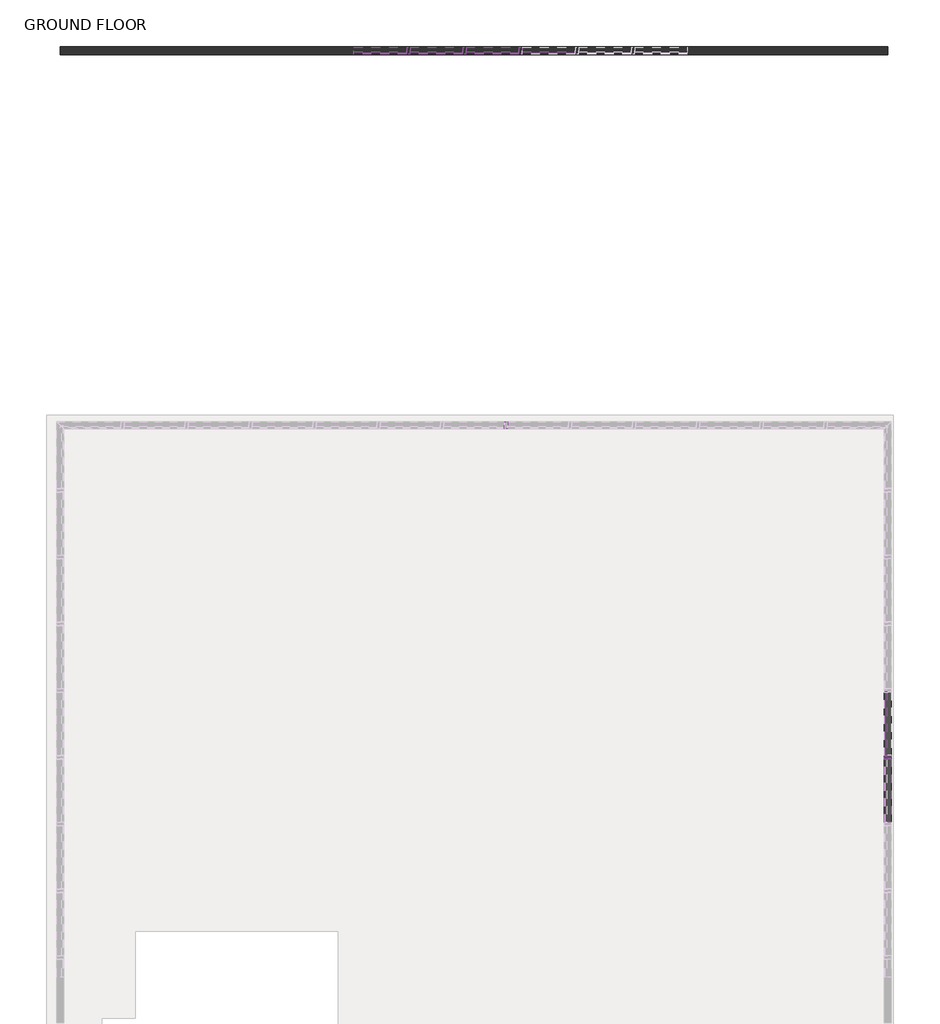
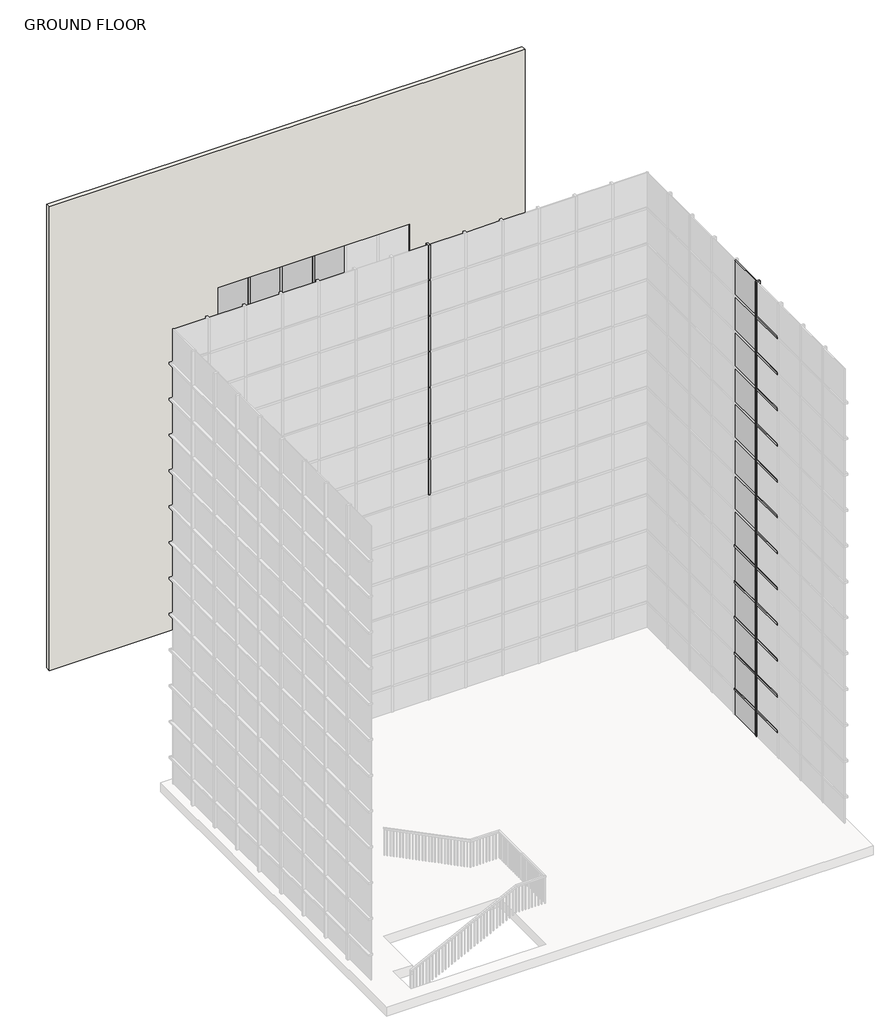
# One storey, part 11 of 16: 82 members, 45 plates, 1 wall.
"""IFC4 building model written with IfcOpenShell, lengths in millimetres."""

from ifc_helpers import new_model, si_unit, frame, origin, place, context, project, spatial, polyline, outline, extrude, transform, mapped, element, save
from components import member_b860638c, member_31fee25f, member_49b1bc66, member_76449a13, member_fdbefc00, member_3df3cfcf, member_368818a6, system_panel_glazed_49652e9e, system_panel_glazed_6a711426

model = new_model("IFC4")

# Units and contexts
model_context = context("Model", 3, world=origin())
ifc_project = project(units=[si_unit("LENGTHUNIT", "METRE", prefix="MILLI")], contexts=[model_context])

# Site, building, storey
site = spatial("IfcSite", under=ifc_project)
building = spatial("IfcBuilding", under=site)
storey = spatial("IfcBuildingStorey", under=building, Name="GROUND FLOOR", Elevation=0.0)

# Members
placement = place(None, origin())
member_shape = member_b860638c(model_context)
element("IfcMember", 1, ObjectType="Rectangular Mullion : 2.5\" x 5\" rectangular", at=placement, inside=storey, context=model_context, shape_type="MappedRepresentation", body=[
    mapped(member_shape, transform((5962.6982466, 315.5011968, 0.0), x_axis=(0.0, 1.0, 0.0), y_axis=(1.0, 0.0, 0.0), z_axis=(0.0, 0.0, -1.0))),
])
member_2_shape = member_31fee25f(model_context)
element("IfcMember", 2, ObjectType="Rectangular Mullion : 2.5\" x 5\" rectangular", at=placement, inside=storey, context=model_context, shape_type="MappedRepresentation", body=[
    mapped(member_2_shape, transform((5962.6982466, 315.5011968, 1168.8884615), x_axis=(0.0, 1.0, 0.0), y_axis=(1.0, 0.0, 0.0), z_axis=(0.0, 0.0, -1.0))),
])
element("IfcMember", 3, ObjectType="Rectangular Mullion : 2.5\" x 5\" rectangular", at=placement, inside=storey, context=model_context, shape_type="MappedRepresentation", body=[
    mapped(member_2_shape, transform((5962.6982466, 315.5011968, 2369.5269231), x_axis=(0.0, 1.0, 0.0), y_axis=(1.0, 0.0, 0.0), z_axis=(0.0, 0.0, -1.0))),
])
element("IfcMember", 4, ObjectType="Rectangular Mullion : 2.5\" x 5\" rectangular", at=placement, inside=storey, context=model_context, shape_type="MappedRepresentation", body=[
    mapped(member_2_shape, transform((5962.6982466, 315.5011968, 3570.1653846), x_axis=(0.0, 1.0, 0.0), y_axis=(1.0, 0.0, 0.0), z_axis=(0.0, 0.0, -1.0))),
])
element("IfcMember", 5, ObjectType="Rectangular Mullion : 2.5\" x 5\" rectangular", at=placement, inside=storey, context=model_context, shape_type="MappedRepresentation", body=[
    mapped(member_2_shape, transform((5962.6982466, 315.5011968, 4770.8038462), x_axis=(0.0, 1.0, 0.0), y_axis=(1.0, 0.0, 0.0), z_axis=(0.0, 0.0, -1.0))),
])
element("IfcMember", 6, ObjectType="Rectangular Mullion : 2.5\" x 5\" rectangular", at=placement, inside=storey, context=model_context, shape_type="MappedRepresentation", body=[
    mapped(member_2_shape, transform((5962.6982466, 315.5011968, 5971.4423077), x_axis=(0.0, 1.0, 0.0), y_axis=(1.0, 0.0, 0.0), z_axis=(0.0, 0.0, -1.0))),
])
element("IfcMember", 7, ObjectType="Rectangular Mullion : 2.5\" x 5\" rectangular", at=placement, inside=storey, context=model_context, shape_type="MappedRepresentation", body=[
    mapped(member_2_shape, transform((5962.6982466, 315.5011968, 7172.0807692), x_axis=(0.0, 1.0, 0.0), y_axis=(1.0, 0.0, 0.0), z_axis=(0.0, 0.0, -1.0))),
])
element("IfcMember", 8, ObjectType="Rectangular Mullion : 2.5\" x 5\" rectangular", at=placement, inside=storey, context=model_context, shape_type="MappedRepresentation", body=[
    mapped(member_2_shape, transform((5962.6982466, 315.5011968, 8372.7192308), x_axis=(0.0, 1.0, 0.0), y_axis=(1.0, 0.0, 0.0), z_axis=(0.0, 0.0, -1.0))),
])
element("IfcMember", 9, ObjectType="Rectangular Mullion : 2.5\" x 5\" rectangular", at=placement, inside=storey, context=model_context, shape_type="MappedRepresentation", body=[
    mapped(member_2_shape, transform((5962.6982466, 315.5011968, 9573.3576923), x_axis=(0.0, 1.0, 0.0), y_axis=(1.0, 0.0, 0.0), z_axis=(0.0, 0.0, -1.0))),
])
element("IfcMember", 10, ObjectType="Rectangular Mullion : 2.5\" x 5\" rectangular", at=placement, inside=storey, context=model_context, shape_type="MappedRepresentation", body=[
    mapped(member_2_shape, transform((5962.6982466, 315.5011968, 10773.9961538), x_axis=(0.0, 1.0, 0.0), y_axis=(1.0, 0.0, 0.0), z_axis=(0.0, 0.0, -1.0))),
])
element("IfcMember", 11, ObjectType="Rectangular Mullion : 2.5\" x 5\" rectangular", at=placement, inside=storey, context=model_context, shape_type="MappedRepresentation", body=[
    mapped(member_2_shape, transform((5962.6982466, 315.5011968, 11974.6346154), x_axis=(0.0, 1.0, 0.0), y_axis=(1.0, 0.0, 0.0), z_axis=(0.0, 0.0, -1.0))),
])
element("IfcMember", 12, ObjectType="Rectangular Mullion : 2.5\" x 5\" rectangular", at=placement, inside=storey, context=model_context, shape_type="MappedRepresentation", body=[
    mapped(member_2_shape, transform((5962.6982466, 315.5011968, 13175.2730769), x_axis=(0.0, 1.0, 0.0), y_axis=(1.0, 0.0, 0.0), z_axis=(0.0, 0.0, -1.0))),
])
element("IfcMember", 13, ObjectType="Rectangular Mullion : 2.5\" x 5\" rectangular", at=placement, inside=storey, context=model_context, shape_type="MappedRepresentation", body=[
    mapped(member_2_shape, transform((-998.3671381, 6370.2261968, 7172.0807692), x_axis=(-1.0, 0.0, 0.0), y_axis=(0.0, 1.0, 0.0), z_axis=(0.0, 0.0, -1.0))),
])
element("IfcMember", 14, ObjectType="Rectangular Mullion : 2.5\" x 5\" rectangular", at=placement, inside=storey, context=model_context, shape_type="MappedRepresentation", body=[
    mapped(member_2_shape, transform((-998.3671381, 6370.2261968, 8372.7192308), x_axis=(-1.0, 0.0, 0.0), y_axis=(0.0, 1.0, 0.0), z_axis=(0.0, 0.0, -1.0))),
])
element("IfcMember", 15, ObjectType="Rectangular Mullion : 2.5\" x 5\" rectangular", at=placement, inside=storey, context=model_context, shape_type="MappedRepresentation", body=[
    mapped(member_2_shape, transform((-998.3671381, 6370.2261968, 9573.3576923), x_axis=(-1.0, 0.0, 0.0), y_axis=(0.0, 1.0, 0.0), z_axis=(0.0, 0.0, -1.0))),
])
element("IfcMember", 16, ObjectType="Rectangular Mullion : 2.5\" x 5\" rectangular", at=placement, inside=storey, context=model_context, shape_type="MappedRepresentation", body=[
    mapped(member_2_shape, transform((-998.3671381, 6370.2261968, 10773.9961538), x_axis=(-1.0, 0.0, 0.0), y_axis=(0.0, 1.0, 0.0), z_axis=(0.0, 0.0, -1.0))),
])
element("IfcMember", 17, ObjectType="Rectangular Mullion : 2.5\" x 5\" rectangular", at=placement, inside=storey, context=model_context, shape_type="MappedRepresentation", body=[
    mapped(member_2_shape, transform((-998.3671381, 6370.2261968, 11974.6346154), x_axis=(-1.0, 0.0, 0.0), y_axis=(0.0, 1.0, 0.0), z_axis=(0.0, 0.0, -1.0))),
])
element("IfcMember", 18, ObjectType="Rectangular Mullion : 2.5\" x 5\" rectangular", at=placement, inside=storey, context=model_context, shape_type="MappedRepresentation", body=[
    mapped(member_2_shape, transform((-998.3671381, 6370.2261968, 13175.2730769), x_axis=(-1.0, 0.0, 0.0), y_axis=(0.0, 1.0, 0.0), z_axis=(0.0, 0.0, -1.0))),
])
element("IfcMember", 19, ObjectType="Rectangular Mullion : 2.5\" x 5\" rectangular", at=placement, inside=storey, context=model_context, shape_type="MappedRepresentation", body=[
    mapped(member_shape, transform((5962.6982466, 315.5011968, 14375.9115385), x_axis=(0.0, 1.0, 0.0), y_axis=(1.0, 0.0, 0.0), z_axis=(0.0, 0.0, -1.0))),
])
element("IfcMember", 20, ObjectType="Rectangular Mullion : 2.5\" x 5\" rectangular", at=placement, inside=storey, context=model_context, shape_type="MappedRepresentation", body=[
    mapped(member_shape, transform((-998.3671381, 6370.2261968, 14375.9115385), x_axis=(-1.0, 0.0, 0.0), y_axis=(0.0, 1.0, 0.0), z_axis=(0.0, 0.0, -1.0))),
])
member_3_shape = member_49b1bc66(model_context)
element("IfcMember", 21, ObjectType="Rectangular Mullion : 2.5\" x 5\" rectangular", at=placement, inside=storey, context=model_context, shape_type="MappedRepresentation", body=[
    mapped(member_3_shape, transform((5962.6982466, 283.7511968, 1168.8884615), x_axis=(0.0, 0.0, 1.0), y_axis=(1.0, 0.0, 0.0), z_axis=(0.0, 1.0, 0.0))),
])
element("IfcMember", 22, ObjectType="Rectangular Mullion : 2.5\" x 5\" rectangular", at=placement, inside=storey, context=model_context, shape_type="MappedRepresentation", body=[
    mapped(member_3_shape, transform((5962.6982466, 1501.0461967, 1168.8884615), x_axis=(0.0, 0.0, 1.0), y_axis=(1.0, 0.0, 0.0), z_axis=(0.0, 1.0, 0.0))),
])
element("IfcMember", 23, ObjectType="Rectangular Mullion : 2.5\" x 5\" rectangular", at=placement, inside=storey, context=model_context, shape_type="MappedRepresentation", body=[
    mapped(member_3_shape, transform((5962.6982466, 283.7511968, 2369.5269231), x_axis=(0.0, 0.0, 1.0), y_axis=(1.0, 0.0, 0.0), z_axis=(0.0, 1.0, 0.0))),
])
element("IfcMember", 24, ObjectType="Rectangular Mullion : 2.5\" x 5\" rectangular", at=placement, inside=storey, context=model_context, shape_type="MappedRepresentation", body=[
    mapped(member_3_shape, transform((5962.6982466, 1501.0461967, 2369.5269231), x_axis=(0.0, 0.0, 1.0), y_axis=(1.0, 0.0, 0.0), z_axis=(0.0, 1.0, 0.0))),
])
element("IfcMember", 25, ObjectType="Rectangular Mullion : 2.5\" x 5\" rectangular", at=placement, inside=storey, context=model_context, shape_type="MappedRepresentation", body=[
    mapped(member_3_shape, transform((5962.6982466, 283.7511968, 3570.1653846), x_axis=(0.0, 0.0, 1.0), y_axis=(1.0, 0.0, 0.0), z_axis=(0.0, 1.0, 0.0))),
])
element("IfcMember", 26, ObjectType="Rectangular Mullion : 2.5\" x 5\" rectangular", at=placement, inside=storey, context=model_context, shape_type="MappedRepresentation", body=[
    mapped(member_3_shape, transform((5962.6982466, 1501.0461967, 3570.1653846), x_axis=(0.0, 0.0, 1.0), y_axis=(1.0, 0.0, 0.0), z_axis=(0.0, 1.0, 0.0))),
])
element("IfcMember", 27, ObjectType="Rectangular Mullion : 2.5\" x 5\" rectangular", at=placement, inside=storey, context=model_context, shape_type="MappedRepresentation", body=[
    mapped(member_3_shape, transform((5962.6982466, 283.7511968, 4770.8038462), x_axis=(0.0, 0.0, 1.0), y_axis=(1.0, 0.0, 0.0), z_axis=(0.0, 1.0, 0.0))),
])
element("IfcMember", 28, ObjectType="Rectangular Mullion : 2.5\" x 5\" rectangular", at=placement, inside=storey, context=model_context, shape_type="MappedRepresentation", body=[
    mapped(member_3_shape, transform((5962.6982466, 1501.0461967, 4770.8038462), x_axis=(0.0, 0.0, 1.0), y_axis=(1.0, 0.0, 0.0), z_axis=(0.0, 1.0, 0.0))),
])
element("IfcMember", 29, ObjectType="Rectangular Mullion : 2.5\" x 5\" rectangular", at=placement, inside=storey, context=model_context, shape_type="MappedRepresentation", body=[
    mapped(member_3_shape, transform((5962.6982466, 283.7511968, 5971.4423077), x_axis=(0.0, 0.0, 1.0), y_axis=(1.0, 0.0, 0.0), z_axis=(0.0, 1.0, 0.0))),
])
element("IfcMember", 30, ObjectType="Rectangular Mullion : 2.5\" x 5\" rectangular", at=placement, inside=storey, context=model_context, shape_type="MappedRepresentation", body=[
    mapped(member_3_shape, transform((5962.6982466, 1501.0461967, 5971.4423077), x_axis=(0.0, 0.0, 1.0), y_axis=(1.0, 0.0, 0.0), z_axis=(0.0, 1.0, 0.0))),
])
element("IfcMember", 31, ObjectType="Rectangular Mullion : 2.5\" x 5\" rectangular", at=placement, inside=storey, context=model_context, shape_type="MappedRepresentation", body=[
    mapped(member_3_shape, transform((5962.6982466, 283.7511968, 7172.0807692), x_axis=(0.0, 0.0, 1.0), y_axis=(1.0, 0.0, 0.0), z_axis=(0.0, 1.0, 0.0))),
])
element("IfcMember", 32, ObjectType="Rectangular Mullion : 2.5\" x 5\" rectangular", at=placement, inside=storey, context=model_context, shape_type="MappedRepresentation", body=[
    mapped(member_3_shape, transform((5962.6982466, 283.7511968, 8372.7192308), x_axis=(0.0, 0.0, 1.0), y_axis=(1.0, 0.0, 0.0), z_axis=(0.0, 1.0, 0.0))),
])
element("IfcMember", 33, ObjectType="Rectangular Mullion : 2.5\" x 5\" rectangular", at=placement, inside=storey, context=model_context, shape_type="MappedRepresentation", body=[
    mapped(member_3_shape, transform((5962.6982466, 283.7511968, 9573.3576923), x_axis=(0.0, 0.0, 1.0), y_axis=(1.0, 0.0, 0.0), z_axis=(0.0, 1.0, 0.0))),
])
element("IfcMember", 34, ObjectType="Rectangular Mullion : 2.5\" x 5\" rectangular", at=placement, inside=storey, context=model_context, shape_type="MappedRepresentation", body=[
    mapped(member_3_shape, transform((5962.6982466, 283.7511968, 10773.9961538), x_axis=(0.0, 0.0, 1.0), y_axis=(1.0, 0.0, 0.0), z_axis=(0.0, 1.0, 0.0))),
])
element("IfcMember", 35, ObjectType="Rectangular Mullion : 2.5\" x 5\" rectangular", at=placement, inside=storey, context=model_context, shape_type="MappedRepresentation", body=[
    mapped(member_3_shape, transform((5962.6982466, 283.7511968, 11974.6346154), x_axis=(0.0, 0.0, 1.0), y_axis=(1.0, 0.0, 0.0), z_axis=(0.0, 1.0, 0.0))),
])
element("IfcMember", 36, ObjectType="Rectangular Mullion : 2.5\" x 5\" rectangular", at=placement, inside=storey, context=model_context, shape_type="MappedRepresentation", body=[
    mapped(member_3_shape, transform((5962.6982466, 283.7511968, 13175.2730769), x_axis=(0.0, 0.0, 1.0), y_axis=(1.0, 0.0, 0.0), z_axis=(0.0, 1.0, 0.0))),
])
element("IfcMember", 37, ObjectType="Rectangular Mullion : 2.5\" x 5\" rectangular", at=placement, inside=storey, context=model_context, shape_type="MappedRepresentation", body=[
    mapped(member_3_shape, transform((5962.6982466, 283.7511968, 14375.9115385), x_axis=(0.0, 0.0, 1.0), y_axis=(1.0, 0.0, 0.0), z_axis=(0.0, 1.0, 0.0))),
])
member_4_shape = member_76449a13(model_context)
element("IfcMember", 38, ObjectType="Rectangular Mullion : 2.5\" x 5\" rectangular", at=placement, inside=storey, context=model_context, shape_type="MappedRepresentation", body=[
    mapped(member_4_shape, transform((-765.2355616, 13200.7626438, 3045.6877023), x_axis=(0.0, 0.0, 1.0), y_axis=(0.0, -1.0, 0.0), z_axis=(1.0, 0.0, 0.0))),
])
element("IfcMember", 39, ObjectType="Rectangular Mullion : 2.5\" x 5\" rectangular", at=placement, inside=storey, context=model_context, shape_type="MappedRepresentation", body=[
    mapped(member_4_shape, transform((-765.2355616, 13200.7626438, 4181.5290519), x_axis=(0.0, 0.0, 1.0), y_axis=(0.0, -1.0, 0.0), z_axis=(1.0, 0.0, 0.0))),
])
element("IfcMember", 40, ObjectType="Rectangular Mullion : 2.5\" x 5\" rectangular", at=placement, inside=storey, context=model_context, shape_type="MappedRepresentation", body=[
    mapped(member_4_shape, transform((-765.2355616, 13200.7626438, 5317.3704015), x_axis=(0.0, 0.0, 1.0), y_axis=(0.0, -1.0, 0.0), z_axis=(1.0, 0.0, 0.0))),
])
element("IfcMember", 41, ObjectType="Rectangular Mullion : 2.5\" x 5\" rectangular", at=placement, inside=storey, context=model_context, shape_type="MappedRepresentation", body=[
    mapped(member_4_shape, transform((-765.2355616, 13200.7626438, 6453.2117511), x_axis=(0.0, 0.0, 1.0), y_axis=(0.0, -1.0, 0.0), z_axis=(1.0, 0.0, 0.0))),
])
element("IfcMember", 42, ObjectType="Rectangular Mullion : 2.5\" x 5\" rectangular", at=placement, inside=storey, context=model_context, shape_type="MappedRepresentation", body=[
    mapped(member_4_shape, transform((-765.2355616, 13200.7626438, 7589.0531007), x_axis=(0.0, 0.0, 1.0), y_axis=(0.0, -1.0, 0.0), z_axis=(1.0, 0.0, 0.0))),
])
element("IfcMember", 43, ObjectType="Rectangular Mullion : 2.5\" x 5\" rectangular", at=placement, inside=storey, context=model_context, shape_type="MappedRepresentation", body=[
    mapped(member_4_shape, transform((-765.2355616, 13200.7626438, 8724.8944503), x_axis=(0.0, 0.0, 1.0), y_axis=(0.0, -1.0, 0.0), z_axis=(1.0, 0.0, 0.0))),
])
element("IfcMember", 44, ObjectType="Rectangular Mullion : 2.5\" x 5\" rectangular", at=placement, inside=storey, context=model_context, shape_type="MappedRepresentation", body=[
    mapped(member_4_shape, transform((-765.2355616, 13200.7626438, 9860.7357999), x_axis=(0.0, 0.0, 1.0), y_axis=(0.0, -1.0, 0.0), z_axis=(1.0, 0.0, 0.0))),
])
element("IfcMember", 45, ObjectType="Rectangular Mullion : 2.5\" x 5\" rectangular", at=placement, inside=storey, context=model_context, shape_type="MappedRepresentation", body=[
    mapped(member_4_shape, transform((-1789.1290689, 13200.7626438, 3045.6877023), x_axis=(0.0, 0.0, 1.0), y_axis=(0.0, -1.0, 0.0), z_axis=(1.0, 0.0, 0.0))),
])
element("IfcMember", 46, ObjectType="Rectangular Mullion : 2.5\" x 5\" rectangular", at=placement, inside=storey, context=model_context, shape_type="MappedRepresentation", body=[
    mapped(member_4_shape, transform((-1789.1290689, 13200.7626438, 4181.5290519), x_axis=(0.0, 0.0, 1.0), y_axis=(0.0, -1.0, 0.0), z_axis=(1.0, 0.0, 0.0))),
])
element("IfcMember", 47, ObjectType="Rectangular Mullion : 2.5\" x 5\" rectangular", at=placement, inside=storey, context=model_context, shape_type="MappedRepresentation", body=[
    mapped(member_4_shape, transform((-1789.1290689, 13200.7626438, 5317.3704015), x_axis=(0.0, 0.0, 1.0), y_axis=(0.0, -1.0, 0.0), z_axis=(1.0, 0.0, 0.0))),
])
element("IfcMember", 48, ObjectType="Rectangular Mullion : 2.5\" x 5\" rectangular", at=placement, inside=storey, context=model_context, shape_type="MappedRepresentation", body=[
    mapped(member_4_shape, transform((-1789.1290689, 13200.7626438, 6453.2117511), x_axis=(0.0, 0.0, 1.0), y_axis=(0.0, -1.0, 0.0), z_axis=(1.0, 0.0, 0.0))),
])
element("IfcMember", 49, ObjectType="Rectangular Mullion : 2.5\" x 5\" rectangular", at=placement, inside=storey, context=model_context, shape_type="MappedRepresentation", body=[
    mapped(member_4_shape, transform((-1789.1290689, 13200.7626438, 7589.0531007), x_axis=(0.0, 0.0, 1.0), y_axis=(0.0, -1.0, 0.0), z_axis=(1.0, 0.0, 0.0))),
])
element("IfcMember", 50, ObjectType="Rectangular Mullion : 2.5\" x 5\" rectangular", at=placement, inside=storey, context=model_context, shape_type="MappedRepresentation", body=[
    mapped(member_4_shape, transform((-1789.1290689, 13200.7626438, 8724.8944503), x_axis=(0.0, 0.0, 1.0), y_axis=(0.0, -1.0, 0.0), z_axis=(1.0, 0.0, 0.0))),
])
element("IfcMember", 51, ObjectType="Rectangular Mullion : 2.5\" x 5\" rectangular", at=placement, inside=storey, context=model_context, shape_type="MappedRepresentation", body=[
    mapped(member_4_shape, transform((-1789.1290689, 13200.7626438, 9860.7357999), x_axis=(0.0, 0.0, 1.0), y_axis=(0.0, -1.0, 0.0), z_axis=(1.0, 0.0, 0.0))),
])
member_5_shape = member_fdbefc00(model_context)
element("IfcMember", 52, ObjectType="Rectangular Mullion : 2.5\" x 5\" rectangular", at=placement, inside=storey, context=model_context, shape_type="MappedRepresentation", body=[
    mapped(member_5_shape, transform((-2813.0225763, 13200.7626438, 3045.6877023), x_axis=(0.0, 0.0, 1.0), y_axis=(0.0, -1.0, 0.0), z_axis=(1.0, 0.0, 0.0))),
])
element("IfcMember", 53, ObjectType="Rectangular Mullion : 2.5\" x 5\" rectangular", at=placement, inside=storey, context=model_context, shape_type="MappedRepresentation", body=[
    mapped(member_5_shape, transform((-2813.0225763, 13200.7626438, 4181.5290519), x_axis=(0.0, 0.0, 1.0), y_axis=(0.0, -1.0, 0.0), z_axis=(1.0, 0.0, 0.0))),
])
element("IfcMember", 54, ObjectType="Rectangular Mullion : 2.5\" x 5\" rectangular", at=placement, inside=storey, context=model_context, shape_type="MappedRepresentation", body=[
    mapped(member_5_shape, transform((-2813.0225763, 13200.7626438, 5317.3704015), x_axis=(0.0, 0.0, 1.0), y_axis=(0.0, -1.0, 0.0), z_axis=(1.0, 0.0, 0.0))),
])
element("IfcMember", 55, ObjectType="Rectangular Mullion : 2.5\" x 5\" rectangular", at=placement, inside=storey, context=model_context, shape_type="MappedRepresentation", body=[
    mapped(member_5_shape, transform((-2813.0225763, 13200.7626438, 6453.2117511), x_axis=(0.0, 0.0, 1.0), y_axis=(0.0, -1.0, 0.0), z_axis=(1.0, 0.0, 0.0))),
])
element("IfcMember", 56, ObjectType="Rectangular Mullion : 2.5\" x 5\" rectangular", at=placement, inside=storey, context=model_context, shape_type="MappedRepresentation", body=[
    mapped(member_5_shape, transform((-2813.0225763, 13200.7626438, 7589.0531007), x_axis=(0.0, 0.0, 1.0), y_axis=(0.0, -1.0, 0.0), z_axis=(1.0, 0.0, 0.0))),
])
element("IfcMember", 57, ObjectType="Rectangular Mullion : 2.5\" x 5\" rectangular", at=placement, inside=storey, context=model_context, shape_type="MappedRepresentation", body=[
    mapped(member_5_shape, transform((-2813.0225763, 13200.7626438, 8724.8944503), x_axis=(0.0, 0.0, 1.0), y_axis=(0.0, -1.0, 0.0), z_axis=(1.0, 0.0, 0.0))),
])
element("IfcMember", 58, ObjectType="Rectangular Mullion : 2.5\" x 5\" rectangular", at=placement, inside=storey, context=model_context, shape_type="MappedRepresentation", body=[
    mapped(member_5_shape, transform((-2813.0225763, 13200.7626438, 9860.7357999), x_axis=(0.0, 0.0, 1.0), y_axis=(0.0, -1.0, 0.0), z_axis=(1.0, 0.0, 0.0))),
])
member_6_shape = member_3df3cfcf(model_context)
element("IfcMember", 59, ObjectType="Rectangular Mullion : 2.5\" x 5\" rectangular", at=placement, inside=storey, context=model_context, shape_type="MappedRepresentation", body=[
    mapped(member_6_shape, transform((-1757.3790689, 13200.7626438, 1941.5963527), x_axis=(1.0, 0.0, 0.0), y_axis=(0.0, -1.0, 0.0), z_axis=(0.0, 0.0, -1.0))),
])
element("IfcMember", 60, ObjectType="Rectangular Mullion : 2.5\" x 5\" rectangular", at=placement, inside=storey, context=model_context, shape_type="MappedRepresentation", body=[
    mapped(member_6_shape, transform((-733.4855616, 13200.7626438, 1941.5963527), x_axis=(1.0, 0.0, 0.0), y_axis=(0.0, -1.0, 0.0), z_axis=(0.0, 0.0, -1.0))),
])
element("IfcMember", 61, ObjectType="Rectangular Mullion : 2.5\" x 5\" rectangular", at=placement, inside=storey, context=model_context, shape_type="MappedRepresentation", body=[
    mapped(member_6_shape, transform((-2781.2725763, 13200.7626438, 1941.5963527), x_axis=(1.0, 0.0, 0.0), y_axis=(0.0, -1.0, 0.0), z_axis=(0.0, 0.0, -1.0))),
])
member_7_shape = member_368818a6(model_context)
element("IfcMember", 62, ObjectType="Rectangular Mullion : 2.5\" x 5\" rectangular", at=placement, inside=storey, context=model_context, shape_type="MappedRepresentation", body=[
    mapped(member_7_shape, transform((-1757.3790689, 13200.7626438, 3045.6877023), x_axis=(1.0, 0.0, 0.0), y_axis=(0.0, -1.0, 0.0), z_axis=(0.0, 0.0, -1.0))),
])
element("IfcMember", 63, ObjectType="Rectangular Mullion : 2.5\" x 5\" rectangular", at=placement, inside=storey, context=model_context, shape_type="MappedRepresentation", body=[
    mapped(member_7_shape, transform((-733.4855616, 13200.7626438, 3045.6877023), x_axis=(1.0, 0.0, 0.0), y_axis=(0.0, -1.0, 0.0), z_axis=(0.0, 0.0, -1.0))),
])
element("IfcMember", 64, ObjectType="Rectangular Mullion : 2.5\" x 5\" rectangular", at=placement, inside=storey, context=model_context, shape_type="MappedRepresentation", body=[
    mapped(member_7_shape, transform((-1757.3790689, 13200.7626438, 4181.5290519), x_axis=(1.0, 0.0, 0.0), y_axis=(0.0, -1.0, 0.0), z_axis=(0.0, 0.0, -1.0))),
])
element("IfcMember", 65, ObjectType="Rectangular Mullion : 2.5\" x 5\" rectangular", at=placement, inside=storey, context=model_context, shape_type="MappedRepresentation", body=[
    mapped(member_7_shape, transform((-733.4855616, 13200.7626438, 4181.5290519), x_axis=(1.0, 0.0, 0.0), y_axis=(0.0, -1.0, 0.0), z_axis=(0.0, 0.0, -1.0))),
])
element("IfcMember", 66, ObjectType="Rectangular Mullion : 2.5\" x 5\" rectangular", at=placement, inside=storey, context=model_context, shape_type="MappedRepresentation", body=[
    mapped(member_7_shape, transform((-1757.3790689, 13200.7626438, 5317.3704015), x_axis=(1.0, 0.0, 0.0), y_axis=(0.0, -1.0, 0.0), z_axis=(0.0, 0.0, -1.0))),
])
element("IfcMember", 67, ObjectType="Rectangular Mullion : 2.5\" x 5\" rectangular", at=placement, inside=storey, context=model_context, shape_type="MappedRepresentation", body=[
    mapped(member_7_shape, transform((-733.4855616, 13200.7626438, 5317.3704015), x_axis=(1.0, 0.0, 0.0), y_axis=(0.0, -1.0, 0.0), z_axis=(0.0, 0.0, -1.0))),
])
element("IfcMember", 68, ObjectType="Rectangular Mullion : 2.5\" x 5\" rectangular", at=placement, inside=storey, context=model_context, shape_type="MappedRepresentation", body=[
    mapped(member_7_shape, transform((-1757.3790689, 13200.7626438, 6453.2117511), x_axis=(1.0, 0.0, 0.0), y_axis=(0.0, -1.0, 0.0), z_axis=(0.0, 0.0, -1.0))),
])
element("IfcMember", 69, ObjectType="Rectangular Mullion : 2.5\" x 5\" rectangular", at=placement, inside=storey, context=model_context, shape_type="MappedRepresentation", body=[
    mapped(member_7_shape, transform((-733.4855616, 13200.7626438, 6453.2117511), x_axis=(1.0, 0.0, 0.0), y_axis=(0.0, -1.0, 0.0), z_axis=(0.0, 0.0, -1.0))),
])
element("IfcMember", 70, ObjectType="Rectangular Mullion : 2.5\" x 5\" rectangular", at=placement, inside=storey, context=model_context, shape_type="MappedRepresentation", body=[
    mapped(member_7_shape, transform((-1757.3790689, 13200.7626438, 7589.0531007), x_axis=(1.0, 0.0, 0.0), y_axis=(0.0, -1.0, 0.0), z_axis=(0.0, 0.0, -1.0))),
])
element("IfcMember", 71, ObjectType="Rectangular Mullion : 2.5\" x 5\" rectangular", at=placement, inside=storey, context=model_context, shape_type="MappedRepresentation", body=[
    mapped(member_7_shape, transform((-733.4855616, 13200.7626438, 7589.0531007), x_axis=(1.0, 0.0, 0.0), y_axis=(0.0, -1.0, 0.0), z_axis=(0.0, 0.0, -1.0))),
])
element("IfcMember", 72, ObjectType="Rectangular Mullion : 2.5\" x 5\" rectangular", at=placement, inside=storey, context=model_context, shape_type="MappedRepresentation", body=[
    mapped(member_7_shape, transform((-1757.3790689, 13200.7626438, 8724.8944503), x_axis=(1.0, 0.0, 0.0), y_axis=(0.0, -1.0, 0.0), z_axis=(0.0, 0.0, -1.0))),
])
element("IfcMember", 73, ObjectType="Rectangular Mullion : 2.5\" x 5\" rectangular", at=placement, inside=storey, context=model_context, shape_type="MappedRepresentation", body=[
    mapped(member_7_shape, transform((-733.4855616, 13200.7626438, 8724.8944503), x_axis=(1.0, 0.0, 0.0), y_axis=(0.0, -1.0, 0.0), z_axis=(0.0, 0.0, -1.0))),
])
element("IfcMember", 74, ObjectType="Rectangular Mullion : 2.5\" x 5\" rectangular", at=placement, inside=storey, context=model_context, shape_type="MappedRepresentation", body=[
    mapped(member_7_shape, transform((-2781.2725763, 13200.7626438, 3045.6877023), x_axis=(1.0, 0.0, 0.0), y_axis=(0.0, -1.0, 0.0), z_axis=(0.0, 0.0, -1.0))),
])
element("IfcMember", 75, ObjectType="Rectangular Mullion : 2.5\" x 5\" rectangular", at=placement, inside=storey, context=model_context, shape_type="MappedRepresentation", body=[
    mapped(member_7_shape, transform((-2781.2725763, 13200.7626438, 4181.5290519), x_axis=(1.0, 0.0, 0.0), y_axis=(0.0, -1.0, 0.0), z_axis=(0.0, 0.0, -1.0))),
])
element("IfcMember", 76, ObjectType="Rectangular Mullion : 2.5\" x 5\" rectangular", at=placement, inside=storey, context=model_context, shape_type="MappedRepresentation", body=[
    mapped(member_7_shape, transform((-2781.2725763, 13200.7626438, 5317.3704015), x_axis=(1.0, 0.0, 0.0), y_axis=(0.0, -1.0, 0.0), z_axis=(0.0, 0.0, -1.0))),
])
element("IfcMember", 77, ObjectType="Rectangular Mullion : 2.5\" x 5\" rectangular", at=placement, inside=storey, context=model_context, shape_type="MappedRepresentation", body=[
    mapped(member_7_shape, transform((-2781.2725763, 13200.7626438, 6453.2117511), x_axis=(1.0, 0.0, 0.0), y_axis=(0.0, -1.0, 0.0), z_axis=(0.0, 0.0, -1.0))),
])
element("IfcMember", 78, ObjectType="Rectangular Mullion : 2.5\" x 5\" rectangular", at=placement, inside=storey, context=model_context, shape_type="MappedRepresentation", body=[
    mapped(member_7_shape, transform((-2781.2725763, 13200.7626438, 7589.0531007), x_axis=(1.0, 0.0, 0.0), y_axis=(0.0, -1.0, 0.0), z_axis=(0.0, 0.0, -1.0))),
])
element("IfcMember", 79, ObjectType="Rectangular Mullion : 2.5\" x 5\" rectangular", at=placement, inside=storey, context=model_context, shape_type="MappedRepresentation", body=[
    mapped(member_7_shape, transform((-2781.2725763, 13200.7626438, 8724.8944503), x_axis=(1.0, 0.0, 0.0), y_axis=(0.0, -1.0, 0.0), z_axis=(0.0, 0.0, -1.0))),
])
element("IfcMember", 80, ObjectType="Rectangular Mullion : 2.5\" x 5\" rectangular", at=placement, inside=storey, context=model_context, shape_type="MappedRepresentation", body=[
    mapped(member_6_shape, transform((-1757.3790689, 13200.7626438, 9860.7357999), x_axis=(1.0, 0.0, 0.0), y_axis=(0.0, -1.0, 0.0), z_axis=(0.0, 0.0, -1.0))),
])
element("IfcMember", 81, ObjectType="Rectangular Mullion : 2.5\" x 5\" rectangular", at=placement, inside=storey, context=model_context, shape_type="MappedRepresentation", body=[
    mapped(member_6_shape, transform((-733.4855616, 13200.7626438, 9860.7357999), x_axis=(1.0, 0.0, 0.0), y_axis=(0.0, -1.0, 0.0), z_axis=(0.0, 0.0, -1.0))),
])
element("IfcMember", 82, ObjectType="Rectangular Mullion : 2.5\" x 5\" rectangular", at=placement, inside=storey, context=model_context, shape_type="MappedRepresentation", body=[
    mapped(member_6_shape, transform((-2781.2725763, 13200.7626438, 9860.7357999), x_axis=(1.0, 0.0, 0.0), y_axis=(0.0, -1.0, 0.0), z_axis=(0.0, 0.0, -1.0))),
])

# Plates
system_panel_glazed_shape = system_panel_glazed_49652e9e(model_context)
element("IfcPlate", 83, ObjectType="System Panel : Glazed", at=placement, inside=storey, context=model_context, shape_type="MappedRepresentation", body=[
    mapped(system_panel_glazed_shape, transform((5962.6982466, 924.1486967, 0.0), x_axis=(0.0, 1.0, 0.0), y_axis=(-1.0, 0.0, 0.0), z_axis=(0.0, 0.0, 1.0))),
])
element("IfcPlate", 84, ObjectType="System Panel : Glazed", at=placement, inside=storey, context=model_context, shape_type="MappedRepresentation", body=[
    mapped(system_panel_glazed_shape, transform((5962.6982466, 924.1486967, 1200.6384615), x_axis=(0.0, 1.0, 0.0), y_axis=(-1.0, 0.0, 0.0), z_axis=(0.0, 0.0, 1.0))),
])
element("IfcPlate", 85, ObjectType="System Panel : Glazed", at=placement, inside=storey, context=model_context, shape_type="MappedRepresentation", body=[
    mapped(system_panel_glazed_shape, transform((5962.6982466, 924.1486967, 2401.2769231), x_axis=(0.0, 1.0, 0.0), y_axis=(-1.0, 0.0, 0.0), z_axis=(0.0, 0.0, 1.0))),
])
element("IfcPlate", 86, ObjectType="System Panel : Glazed", at=placement, inside=storey, context=model_context, shape_type="MappedRepresentation", body=[
    mapped(system_panel_glazed_shape, transform((5962.6982466, 924.1486967, 3601.9153846), x_axis=(0.0, 1.0, 0.0), y_axis=(-1.0, 0.0, 0.0), z_axis=(0.0, 0.0, 1.0))),
])
element("IfcPlate", 87, ObjectType="System Panel : Glazed", at=placement, inside=storey, context=model_context, shape_type="MappedRepresentation", body=[
    mapped(system_panel_glazed_shape, transform((5962.6982466, 924.1486967, 4802.5538462), x_axis=(0.0, 1.0, 0.0), y_axis=(-1.0, 0.0, 0.0), z_axis=(0.0, 0.0, 1.0))),
])
element("IfcPlate", 88, ObjectType="System Panel : Glazed", at=placement, inside=storey, context=model_context, shape_type="MappedRepresentation", body=[
    mapped(system_panel_glazed_shape, transform((5962.6982466, 924.1486967, 6003.1923077), x_axis=(0.0, 1.0, 0.0), y_axis=(-1.0, 0.0, 0.0), z_axis=(0.0, 0.0, 1.0))),
])
element("IfcPlate", 89, ObjectType="System Panel : Glazed", at=placement, inside=storey, context=model_context, shape_type="MappedRepresentation", body=[
    mapped(system_panel_glazed_shape, transform((5962.6982466, 924.1486967, 7203.8307692), x_axis=(0.0, 1.0, 0.0), y_axis=(-1.0, 0.0, 0.0), z_axis=(0.0, 0.0, 1.0))),
])
element("IfcPlate", 90, ObjectType="System Panel : Glazed", at=placement, inside=storey, context=model_context, shape_type="MappedRepresentation", body=[
    mapped(system_panel_glazed_shape, transform((5962.6982466, 924.1486967, 8404.4692308), x_axis=(0.0, 1.0, 0.0), y_axis=(-1.0, 0.0, 0.0), z_axis=(0.0, 0.0, 1.0))),
])
element("IfcPlate", 91, ObjectType="System Panel : Glazed", at=placement, inside=storey, context=model_context, shape_type="MappedRepresentation", body=[
    mapped(system_panel_glazed_shape, transform((5962.6982466, 924.1486967, 9605.1076923), x_axis=(0.0, 1.0, 0.0), y_axis=(-1.0, 0.0, 0.0), z_axis=(0.0, 0.0, 1.0))),
])
element("IfcPlate", 92, ObjectType="System Panel : Glazed", at=placement, inside=storey, context=model_context, shape_type="MappedRepresentation", body=[
    mapped(system_panel_glazed_shape, transform((5962.6982466, 924.1486967, 10805.7461538), x_axis=(0.0, 1.0, 0.0), y_axis=(-1.0, 0.0, 0.0), z_axis=(0.0, 0.0, 1.0))),
])
element("IfcPlate", 93, ObjectType="System Panel : Glazed", at=placement, inside=storey, context=model_context, shape_type="MappedRepresentation", body=[
    mapped(system_panel_glazed_shape, transform((5962.6982466, 924.1486967, 12006.3846154), x_axis=(0.0, 1.0, 0.0), y_axis=(-1.0, 0.0, 0.0), z_axis=(0.0, 0.0, 1.0))),
])
element("IfcPlate", 94, ObjectType="System Panel : Glazed", at=placement, inside=storey, context=model_context, shape_type="MappedRepresentation", body=[
    mapped(system_panel_glazed_shape, transform((5962.6982466, 924.1486967, 13207.0230769), x_axis=(0.0, 1.0, 0.0), y_axis=(-1.0, 0.0, 0.0), z_axis=(0.0, 0.0, 1.0))),
])
element("IfcPlate", 95, ObjectType="System Panel : Glazed", at=placement, inside=storey, context=model_context, shape_type="MappedRepresentation", body=[
    mapped(system_panel_glazed_shape, transform((5962.6982466, 924.1486967, 14407.6615385), x_axis=(0.0, 1.0, 0.0), y_axis=(-1.0, 0.0, 0.0), z_axis=(0.0, 0.0, 1.0))),
])
system_panel_glazed_2_shape = system_panel_glazed_6a711426(model_context)
element("IfcPlate", 96, ObjectType="System Panel : Glazed", at=placement, inside=storey, context=model_context, shape_type="MappedRepresentation", body=[
    mapped(system_panel_glazed_2_shape, transform((-3293.2193301, 13200.7626438, 1941.5963527), x_axis=(1.0, 0.0, 0.0), y_axis=(0.0, 1.0, 0.0), z_axis=(0.0, 0.0, 1.0))),
])
element("IfcPlate", 97, ObjectType="System Panel : Glazed", at=placement, inside=storey, context=model_context, shape_type="MappedRepresentation", body=[
    mapped(system_panel_glazed_2_shape, transform((-1245.4323153, 13200.7626438, 1941.5963527), x_axis=(1.0, 0.0, 0.0), y_axis=(0.0, 1.0, 0.0), z_axis=(0.0, 0.0, 1.0))),
])
element("IfcPlate", 98, ObjectType="System Panel : Glazed", at=placement, inside=storey, context=model_context, shape_type="MappedRepresentation", body=[
    mapped(system_panel_glazed_2_shape, transform((-221.5388079, 13200.7626438, 1941.5963527), x_axis=(1.0, 0.0, 0.0), y_axis=(0.0, 1.0, 0.0), z_axis=(0.0, 0.0, 1.0))),
])
element("IfcPlate", 99, ObjectType="System Panel : Glazed", at=placement, inside=storey, context=model_context, shape_type="MappedRepresentation", body=[
    mapped(system_panel_glazed_2_shape, transform((-3293.2193301, 13200.7626438, 3077.4377023), x_axis=(1.0, 0.0, 0.0), y_axis=(0.0, 1.0, 0.0), z_axis=(0.0, 0.0, 1.0))),
])
element("IfcPlate", 100, ObjectType="System Panel : Glazed", at=placement, inside=storey, context=model_context, shape_type="MappedRepresentation", body=[
    mapped(system_panel_glazed_2_shape, transform((-1245.4323153, 13200.7626438, 3077.4377023), x_axis=(1.0, 0.0, 0.0), y_axis=(0.0, 1.0, 0.0), z_axis=(0.0, 0.0, 1.0))),
])
element("IfcPlate", 101, ObjectType="System Panel : Glazed", at=placement, inside=storey, context=model_context, shape_type="MappedRepresentation", body=[
    mapped(system_panel_glazed_2_shape, transform((-221.5388079, 13200.7626438, 3077.4377023), x_axis=(1.0, 0.0, 0.0), y_axis=(0.0, 1.0, 0.0), z_axis=(0.0, 0.0, 1.0))),
])
element("IfcPlate", 102, ObjectType="System Panel : Glazed", at=placement, inside=storey, context=model_context, shape_type="MappedRepresentation", body=[
    mapped(system_panel_glazed_2_shape, transform((-3293.2193301, 13200.7626438, 4213.2790519), x_axis=(1.0, 0.0, 0.0), y_axis=(0.0, 1.0, 0.0), z_axis=(0.0, 0.0, 1.0))),
])
element("IfcPlate", 103, ObjectType="System Panel : Glazed", at=placement, inside=storey, context=model_context, shape_type="MappedRepresentation", body=[
    mapped(system_panel_glazed_2_shape, transform((-1245.4323153, 13200.7626438, 4213.2790519), x_axis=(1.0, 0.0, 0.0), y_axis=(0.0, 1.0, 0.0), z_axis=(0.0, 0.0, 1.0))),
])
element("IfcPlate", 104, ObjectType="System Panel : Glazed", at=placement, inside=storey, context=model_context, shape_type="MappedRepresentation", body=[
    mapped(system_panel_glazed_2_shape, transform((-221.5388079, 13200.7626438, 4213.2790519), x_axis=(1.0, 0.0, 0.0), y_axis=(0.0, 1.0, 0.0), z_axis=(0.0, 0.0, 1.0))),
])
element("IfcPlate", 105, ObjectType="System Panel : Glazed", at=placement, inside=storey, context=model_context, shape_type="MappedRepresentation", body=[
    mapped(system_panel_glazed_2_shape, transform((-3293.2193301, 13200.7626438, 5349.1204015), x_axis=(1.0, 0.0, 0.0), y_axis=(0.0, 1.0, 0.0), z_axis=(0.0, 0.0, 1.0))),
])
element("IfcPlate", 106, ObjectType="System Panel : Glazed", at=placement, inside=storey, context=model_context, shape_type="MappedRepresentation", body=[
    mapped(system_panel_glazed_2_shape, transform((-1245.4323153, 13200.7626438, 5349.1204015), x_axis=(1.0, 0.0, 0.0), y_axis=(0.0, 1.0, 0.0), z_axis=(0.0, 0.0, 1.0))),
])
element("IfcPlate", 107, ObjectType="System Panel : Glazed", at=placement, inside=storey, context=model_context, shape_type="MappedRepresentation", body=[
    mapped(system_panel_glazed_2_shape, transform((-221.5388079, 13200.7626438, 5349.1204015), x_axis=(1.0, 0.0, 0.0), y_axis=(0.0, 1.0, 0.0), z_axis=(0.0, 0.0, 1.0))),
])
element("IfcPlate", 108, ObjectType="System Panel : Glazed", at=placement, inside=storey, context=model_context, shape_type="MappedRepresentation", body=[
    mapped(system_panel_glazed_2_shape, transform((-3293.2193301, 13200.7626438, 6484.9617511), x_axis=(1.0, 0.0, 0.0), y_axis=(0.0, 1.0, 0.0), z_axis=(0.0, 0.0, 1.0))),
])
element("IfcPlate", 109, ObjectType="System Panel : Glazed", at=placement, inside=storey, context=model_context, shape_type="MappedRepresentation", body=[
    mapped(system_panel_glazed_2_shape, transform((-1245.4323153, 13200.7626438, 6484.9617511), x_axis=(1.0, 0.0, 0.0), y_axis=(0.0, 1.0, 0.0), z_axis=(0.0, 0.0, 1.0))),
])
element("IfcPlate", 110, ObjectType="System Panel : Glazed", at=placement, inside=storey, context=model_context, shape_type="MappedRepresentation", body=[
    mapped(system_panel_glazed_2_shape, transform((-221.5388079, 13200.7626438, 6484.9617511), x_axis=(1.0, 0.0, 0.0), y_axis=(0.0, 1.0, 0.0), z_axis=(0.0, 0.0, 1.0))),
])
element("IfcPlate", 111, ObjectType="System Panel : Glazed", at=placement, inside=storey, context=model_context, shape_type="MappedRepresentation", body=[
    mapped(system_panel_glazed_2_shape, transform((-3293.2193301, 13200.7626438, 7620.8031007), x_axis=(1.0, 0.0, 0.0), y_axis=(0.0, 1.0, 0.0), z_axis=(0.0, 0.0, 1.0))),
])
element("IfcPlate", 112, ObjectType="System Panel : Glazed", at=placement, inside=storey, context=model_context, shape_type="MappedRepresentation", body=[
    mapped(system_panel_glazed_2_shape, transform((-1245.4323153, 13200.7626438, 7620.8031007), x_axis=(1.0, 0.0, 0.0), y_axis=(0.0, 1.0, 0.0), z_axis=(0.0, 0.0, 1.0))),
])
element("IfcPlate", 113, ObjectType="System Panel : Glazed", at=placement, inside=storey, context=model_context, shape_type="MappedRepresentation", body=[
    mapped(system_panel_glazed_2_shape, transform((-221.5388079, 13200.7626438, 7620.8031007), x_axis=(1.0, 0.0, 0.0), y_axis=(0.0, 1.0, 0.0), z_axis=(0.0, 0.0, 1.0))),
])
element("IfcPlate", 114, ObjectType="System Panel : Glazed", at=placement, inside=storey, context=model_context, shape_type="MappedRepresentation", body=[
    mapped(system_panel_glazed_2_shape, transform((-3293.2193301, 13200.7626438, 8756.6444503), x_axis=(1.0, 0.0, 0.0), y_axis=(0.0, 1.0, 0.0), z_axis=(0.0, 0.0, 1.0))),
])
element("IfcPlate", 115, ObjectType="System Panel : Glazed", at=placement, inside=storey, context=model_context, shape_type="MappedRepresentation", body=[
    mapped(system_panel_glazed_2_shape, transform((-1245.4323153, 13200.7626438, 8756.6444503), x_axis=(1.0, 0.0, 0.0), y_axis=(0.0, 1.0, 0.0), z_axis=(0.0, 0.0, 1.0))),
])
element("IfcPlate", 116, ObjectType="System Panel : Glazed", at=placement, inside=storey, context=model_context, shape_type="MappedRepresentation", body=[
    mapped(system_panel_glazed_2_shape, transform((-221.5388079, 13200.7626438, 8756.6444503), x_axis=(1.0, 0.0, 0.0), y_axis=(0.0, 1.0, 0.0), z_axis=(0.0, 0.0, 1.0))),
])
element("IfcPlate", 117, ObjectType="System Panel : Glazed", at=placement, inside=storey, context=model_context, shape_type="MappedRepresentation", body=[
    mapped(system_panel_glazed_2_shape, transform((-3293.2193301, 13200.7626438, 9892.4857999), x_axis=(1.0, 0.0, 0.0), y_axis=(0.0, 1.0, 0.0), z_axis=(0.0, 0.0, 1.0))),
])
element("IfcPlate", 118, ObjectType="System Panel : Glazed", at=placement, inside=storey, context=model_context, shape_type="MappedRepresentation", body=[
    mapped(system_panel_glazed_2_shape, transform((-1245.4323153, 13200.7626438, 9892.4857999), x_axis=(1.0, 0.0, 0.0), y_axis=(0.0, 1.0, 0.0), z_axis=(0.0, 0.0, 1.0))),
])
element("IfcPlate", 119, ObjectType="System Panel : Glazed", at=placement, inside=storey, context=model_context, shape_type="MappedRepresentation", body=[
    mapped(system_panel_glazed_2_shape, transform((-221.5388079, 13200.7626438, 9892.4857999), x_axis=(1.0, 0.0, 0.0), y_axis=(0.0, 1.0, 0.0), z_axis=(0.0, 0.0, 1.0))),
])
element("IfcPlate", 120, ObjectType="System Panel : Glazed", at=placement, inside=storey, context=model_context, shape_type="MappedRepresentation", body=[
    mapped(system_panel_glazed_2_shape, transform((-2269.3258226, 13200.7626438, 1941.5963527), x_axis=(1.0, 0.0, 0.0), y_axis=(0.0, 1.0, 0.0), z_axis=(0.0, 0.0, 1.0))),
])
element("IfcPlate", 121, ObjectType="System Panel : Glazed", at=placement, inside=storey, context=model_context, shape_type="MappedRepresentation", body=[
    mapped(system_panel_glazed_2_shape, transform((-2269.3258226, 13200.7626438, 3077.4377023), x_axis=(1.0, 0.0, 0.0), y_axis=(0.0, 1.0, 0.0), z_axis=(0.0, 0.0, 1.0))),
])
element("IfcPlate", 122, ObjectType="System Panel : Glazed", at=placement, inside=storey, context=model_context, shape_type="MappedRepresentation", body=[
    mapped(system_panel_glazed_2_shape, transform((-2269.3258226, 13200.7626438, 4213.2790519), x_axis=(1.0, 0.0, 0.0), y_axis=(0.0, 1.0, 0.0), z_axis=(0.0, 0.0, 1.0))),
])
element("IfcPlate", 123, ObjectType="System Panel : Glazed", at=placement, inside=storey, context=model_context, shape_type="MappedRepresentation", body=[
    mapped(system_panel_glazed_2_shape, transform((-2269.3258226, 13200.7626438, 5349.1204015), x_axis=(1.0, 0.0, 0.0), y_axis=(0.0, 1.0, 0.0), z_axis=(0.0, 0.0, 1.0))),
])
element("IfcPlate", 124, ObjectType="System Panel : Glazed", at=placement, inside=storey, context=model_context, shape_type="MappedRepresentation", body=[
    mapped(system_panel_glazed_2_shape, transform((-2269.3258226, 13200.7626438, 6484.9617511), x_axis=(1.0, 0.0, 0.0), y_axis=(0.0, 1.0, 0.0), z_axis=(0.0, 0.0, 1.0))),
])
element("IfcPlate", 125, ObjectType="System Panel : Glazed", at=placement, inside=storey, context=model_context, shape_type="MappedRepresentation", body=[
    mapped(system_panel_glazed_2_shape, transform((-2269.3258226, 13200.7626438, 7620.8031007), x_axis=(1.0, 0.0, 0.0), y_axis=(0.0, 1.0, 0.0), z_axis=(0.0, 0.0, 1.0))),
])
element("IfcPlate", 126, ObjectType="System Panel : Glazed", at=placement, inside=storey, context=model_context, shape_type="MappedRepresentation", body=[
    mapped(system_panel_glazed_2_shape, transform((-2269.3258226, 13200.7626438, 8756.6444503), x_axis=(1.0, 0.0, 0.0), y_axis=(0.0, 1.0, 0.0), z_axis=(0.0, 0.0, 1.0))),
])
element("IfcPlate", 127, ObjectType="System Panel : Glazed", at=placement, inside=storey, context=model_context, shape_type="MappedRepresentation", body=[
    mapped(system_panel_glazed_2_shape, transform((-2269.3258226, 13200.7626438, 9892.4857999), x_axis=(1.0, 0.0, 0.0), y_axis=(0.0, 1.0, 0.0), z_axis=(0.0, 0.0, 1.0))),
])

# Wall
element("IfcWall", 128, ObjectType="Generic - 6\"", at=placement, inside=storey, context=model_context, shape_type="SweptSolid", body=[
    extrude(outline(polyline([(0.0, -9124.9017534), (0.0, 5962.6982466), (15544.8, 5962.6982466), (15544.8, -9124.9017534), (0.0, -9124.9017534)]), holes=[polyline([(10964.8271495, -3773.4160839), (10964.8271495, 2306.4449607), (1941.5963527, 2306.4449607), (1941.5963527, -3773.4160839), (10964.8271495, -3773.4160839)])]), frame((0.0, 13124.5626438, 0.0), z_axis=(0.0, 1.0, 0.0), x_axis=(0.0, 0.0, 1.0)), (0.0, 0.0, 1.0), 152.4),
])

save(model, "model.ifc")

# Revit data of these elements
# Type "Rectangular Mullion : 2.5\" x 5\" rectangular"
#   built-in parameter 1007304 = 0.416667 (stored number, unit not read)
#   built-in parameter 1007301 = 0.104167 (stored number, unit not read)
#   built-in parameter 1007300 = 0.104167 (stored number, unit not read)
# Type "System Panel : Glazed"
#   Construction Type Id = "GSP4R"
#   Analytic Construction = "1/8 in Pilkington single glazing"
#   Visual Light Transmittance = 0.9
#   Solar Heat Gain Coefficient = 0.86
#   Heat Transfer Coefficient (U) = 1.18115 BTU/(h·ft²·°F)
#   Define Thermal Properties by = 1
# Type "Generic - 6\""
#   Assembly Code = "B2010"
#   Layers, outside or top first: 0' - 6" no material (function 1)
# Elements 1, 2, 3, 4, 5, 6, 7, 8, 9, 10, 11, 12, 13, 14, 15, 16, 17, 18, 19, 20, 21, 22, 23, 24, 25, 26, 27, 28, 29, 30, 31, 32, 33, 34, 35, 36, 37, 38, 39, 40, 41, 42, 43, 44, 45, 46, 47, 48, 49, 50, 51, 52, 53, 54, 55, 56, 57, 58, 59, 60, 61, 62, 63, 64, 65, 66, 67, 68, 69, 70, 71, 72, 73, 74, 75, 76, 77, 78, 79, 80, 81, 82 (IfcMember, "Rectangular Mullion : 2.5\" x 5\" rectangular")
#   Phase Created = New Construction
#   Materials on its faces: "Aluminum"
# Elements 83, 84, 85, 86, 87, 88, 89, 90, 91, 92, 93, 94, 95, 96, 97, 98, 99, 100, 101, 102, 103, 104, 105, 106, 107, 108, 109, 110, 111, 112, 113, 114, 115, 116, 117, 118, 119, 120, 121, 122, 123, 124, 125, 126, 127 (IfcPlate, "System Panel : Glazed")
#   Phase Created = New Construction
#   Materials on its faces: "Glass"
# Element 128 (IfcWall, "Generic - 6\"")
#   Top Offset = 11' - 0"
#   Base Offset = 0' - 0"
#   wall height = 51' - 0"
#   Phase Created = New Construction
#   Base Constraint = GROUND FLOOR
#   Top Constraint = ROOF
#   Materials on its faces: "Default Wall"
# Materials
#   "Aluminum": class "Metal", colour RGB 247 247 247, transparency 0, Description = "Aluminum 6061", Cost = 0
#   "Glass": class "Glass", colour RGB 0 128 192, transparency 0.75, Description = "Soda Lime Glass", Cost = 0
#   "Default Wall": colour RGB 128 128 128, transparency 0, Cost = 0
